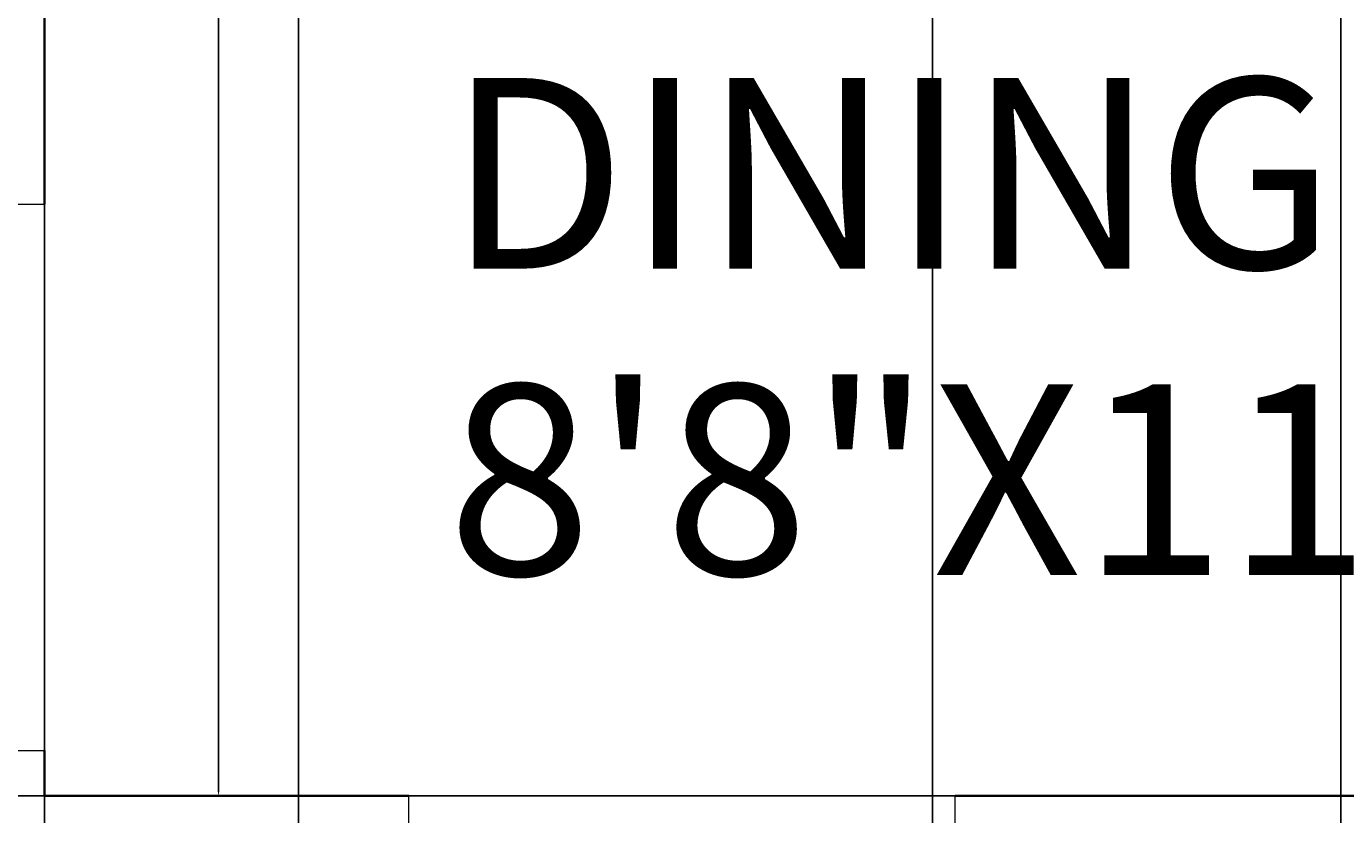
# Model space of a CAD drawing. Units: feet. Extents: x 1654 to 2985, y 1348 to 2230.
# Tile 24 of 53: x 1956 to 2014, y 1750 to 1785. Entities that reach past the tile are written whole.
import ezdxf

# ---------------------------------------------------------------- set-up
doc = ezdxf.new("R2010")
doc.units = ezdxf.units.FT
for name, color, linetype, lineweight in [('A-ANNO-DIMS', 2, 'Continuous', 18), ('A-AREA-IDEN', 7, 'Continuous', 18), ('A-DOOR', 3, 'Continuous', 18), ('A-WALL', 7, 'Continuous', 35)]:
    doc.layers.add(name, color=color, linetype=linetype, lineweight=lineweight)
doc.styles.get("Standard").update_dxf_attribs({"font": 'arial.ttf'})
doc.dimstyles.get("Standard").update_dxf_attribs({"dimtxt": 0.18, "dimasz": 0.18, "dimexe": 0.18, "dimexo": 0.0625, "dimgap": 0.09, "dimtad": 0, "dimtih": 1, "dimtoh": 1, "dimdec": 4, "dimzin": 0, "dimdsep": 46, "dimtxsty": 'Standard', "dimcen": 0.09, "dimadec": 0, "dimazin": 0, "dimtfac": 1, "dimtdec": 4, "dimtofl": 0, "dimtmove": 0, "dimatfit": 3, "dimfxl": 1, "dimtolj": 1, "dimtzin": 0, "dimarcsym": 0})

# ---------------------------------------------------------------- blocks, each defined once
blk = doc.blocks.new('DOOR-INT-SINGLE')
for p, q in [((0, 24), (9, 24)), ((-24, 0), (9, 0))]:
    blk.add_line(p, q)
blk.add_arc((0, 0), 24, 90, 180)
blk = doc.blocks.new('*D74')
at = {"layer": 'A-ANNO-DIMS', "color": 0, "lineweight": -2, "transparency": 16777216}
for p, q in [((1948.155, 1862.255), (1964.922, 1862.255)), ((1964.742, 1862.075), (1964.742, 1806.938)), ((1964.742, 1751.435), (1964.742, 1806.572)), ((1948.155, 1751.255), (1964.922, 1751.255))]:
    blk.add_line(p, q, dxfattribs=at)
at = {"layer": 'A-ANNO-DIMS', "color": 0, "transparency": 16777216}
for points in [[(1964.712, 1862.075), (1964.772, 1862.075), (1964.742, 1862.255)], [(1964.712, 1751.435), (1964.772, 1751.435), (1964.742, 1751.255)]]:
    blk.add_solid(points, dxfattribs=at)
at = {"layer": 'Defpoints', "color": 0, "transparency": 16777216}
for p in [(1948.092, 1862.255), (1964.742, 1862.255), (1948.092, 1751.255)]:
    blk.add_point(p, dxfattribs=at)
at = {"layer": 'A-ANNO-DIMS', "color": 0, "transparency": 16777216, "insert": (1964.742, 1806.755), "char_height": 0.18, "attachment_point": 5}
blk.add_mtext('\\A1;COUNTER 111 TYP.', dxfattribs=at)
blk = doc.blocks.new('*D91')
at = {"layer": 'A-ANNO-DIMS', "color": 0, "lineweight": -2, "transparency": 16777216}
for p, q in [((1852.155, 1801.468), (2242.272, 1801.468)), ((2242.092, 1801.288), (2242.092, 1776.544)), ((2242.092, 1751.435), (2242.092, 1776.18)), ((1852.155, 1751.255), (2242.272, 1751.255))]:
    blk.add_line(p, q, dxfattribs=at)
at = {"layer": 'A-ANNO-DIMS', "color": 0, "transparency": 16777216}
for points in [[(2242.062, 1801.288), (2242.122, 1801.288), (2242.092, 1801.468)], [(2242.062, 1751.435), (2242.122, 1751.435), (2242.092, 1751.255)]]:
    blk.add_solid(points, dxfattribs=at)
at = {"layer": 'Defpoints', "color": 0, "transparency": 16777216}
for p in [(1852.092, 1801.468), (2242.092, 1801.468), (1852.092, 1751.255)]:
    blk.add_point(p, dxfattribs=at)
at = {"layer": 'A-ANNO-DIMS', "color": 0, "transparency": 16777216, "insert": (2242.092, 1776.362), "char_height": 0.18, "attachment_point": 5}
blk.add_mtext('\\A1;50.21', dxfattribs=at)
blk = doc.blocks.new('*D97')
at = {"layer": 'A-ANNO-DIMS', "color": 0, "lineweight": -2, "transparency": 16777216}
for p, q in [((1957.092, 2108.192), (1957.092, 1534.075)), ((1968.254, 2108.192), (1968.254, 1534.075)), ((1957.272, 1534.255), (1962.219, 1534.255)), ((1968.074, 1534.255), (1963.128, 1534.255))]:
    blk.add_line(p, q, dxfattribs=at)
at = {"layer": 'A-ANNO-DIMS', "color": 0, "transparency": 16777216}
for points in [[(1957.272, 1534.285), (1957.272, 1534.225), (1957.092, 1534.255)], [(1968.074, 1534.285), (1968.074, 1534.225), (1968.254, 1534.255)]]:
    blk.add_solid(points, dxfattribs=at)
at = {"layer": 'Defpoints', "color": 0, "transparency": 16777216}
for p in [(1957.092, 2108.255), (1968.254, 2108.255), (1968.254, 1534.255)]:
    blk.add_point(p, dxfattribs=at)
at = {"layer": 'A-ANNO-DIMS', "color": 0, "transparency": 16777216, "insert": (1962.673, 1534.255), "char_height": 0.18, "attachment_point": 5}
blk.add_mtext('\\A1;11.162', dxfattribs=at)
blk = doc.blocks.new('*D98')
at = {"layer": 'A-ANNO-DIMS', "color": 0, "lineweight": -2, "transparency": 16777216}
for p, q in [((2061.03, 1811.081), (1811.912, 1811.081)), ((1812.092, 1810.901), (1812.092, 1781.35)), ((1812.092, 1751.435), (1812.092, 1780.986)), ((2061.03, 1751.255), (1811.912, 1751.255))]:
    blk.add_line(p, q, dxfattribs=at)
at = {"layer": 'A-ANNO-DIMS', "color": 0, "transparency": 16777216}
for points in [[(1812.062, 1810.901), (1812.122, 1810.901), (1812.092, 1811.081)], [(1812.062, 1751.435), (1812.122, 1751.435), (1812.092, 1751.255)]]:
    blk.add_solid(points, dxfattribs=at)
at = {"layer": 'Defpoints', "color": 0, "transparency": 16777216}
for p in [(1812.092, 1811.081), (2061.092, 1811.081), (2061.092, 1751.255)]:
    blk.add_point(p, dxfattribs=at)
at = {"layer": 'A-ANNO-DIMS', "color": 0, "transparency": 16777216, "insert": (1812.092, 1781.168), "char_height": 0.18, "attachment_point": 5}
blk.add_mtext('\\A1;59.83', dxfattribs=at)
blk = doc.blocks.new('*D101')
at = {"layer": 'A-ANNO-DIMS', "color": 0, "lineweight": -2, "transparency": 16777216}
for p, q in [((1996.092, 2039.192), (1996.092, 1534.075)), ((2014.016, 2039.192), (2014.016, 1534.075)), ((1996.272, 1534.255), (2004.599, 1534.255)), ((2013.836, 1534.255), (2005.509, 1534.255))]:
    blk.add_line(p, q, dxfattribs=at)
at = {"layer": 'A-ANNO-DIMS', "color": 0, "transparency": 16777216}
for points in [[(1996.272, 1534.285), (1996.272, 1534.225), (1996.092, 1534.255)], [(2013.836, 1534.285), (2013.836, 1534.225), (2014.016, 1534.255)]]:
    blk.add_solid(points, dxfattribs=at)
at = {"layer": 'Defpoints', "color": 0, "transparency": 16777216}
for p in [(1996.092, 2039.255), (2014.016, 2039.255), (2014.016, 1534.255)]:
    blk.add_point(p, dxfattribs=at)
at = {"layer": 'A-ANNO-DIMS', "color": 0, "transparency": 16777216, "insert": (2005.054, 1534.255), "char_height": 0.18, "attachment_point": 5}
blk.add_mtext('\\A1;17.924', dxfattribs=at)

msp = doc.modelspace()

# ---------------------------------------------------------------- linework, layer by layer
at = {"layer": 'A-WALL'}
for p, q in [((1957.0924, 1777.2549), (1957.0924, 1886.2549)), ((1957.0924, 1751.2549), (1957.0924, 1753.2549)), ((1973.0924, 1751.2549), (1957.0924, 1751.2549)), ((1999.0924, 1751.2549), (1997.0924, 1751.2549)), ((2019.7567, 1751.2549), (1997.0924, 1751.2549))]:
    msp.add_line(p, q, dxfattribs=at)

# ---------------------------------------------------------------- block references
at = {"layer": 'A-DOOR'}
msp.add_blockref('DOOR-INT-SINGLE', (1948.0924, 1753.2549), dxfattribs=at)
at = {"layer": 'A-DOOR', "rotation": 90.00000000000055}
msp.add_blockref('DOOR-INT-SINGLE', (1997.0924, 1742.2549), dxfattribs=at)

# ---------------------------------------------------------------- texts
at = {"layer": 'A-AREA-IDEN'}
for s, p in [('DINING', (1974.793, 1774.4257)), ('8\'8"X11\'3"', (1974.793, 1760.9622))]:
    msp.add_text(s, height=8.38114, dxfattribs=at).set_placement(p)

# ---------------------------------------------------------------- dimensions: what is measured, and where the dimension line sits
at = {"layer": 'A-ANNO-DIMS'}
for base, p1, p2, picture, middle in [((1968.2542, 1534.2549), (1957.0924, 2108.2549), (1968.2542, 2108.2549), '*D97', (1962.6733, 1534.2549)), ((2014.016, 1534.2549), (1996.0924, 2039.2549), (2014.016, 2039.2549), '*D101', (2005.0542, 1534.2549))]:
    dim = msp.add_linear_dim(base=base, p1=p1, p2=p2, dimstyle='Standard', override={"dimdec": 3, "dimlfac": 1, "dimrnd": 0, "dimzin": 0, "dimdsep": 46, "dimlunit": 2}, dxfattribs=at)
    dim.commit()
    dim.dimension.update_dxf_attribs({"geometry": picture, "text_midpoint": middle})
dim = msp.add_linear_dim(base=(1964.7424, 1862.2549), p1=(1948.0924, 1751.2549), p2=(1948.0924, 1862.2549), angle=90, text='COUNTER <> TYP.', dimstyle='Standard', override={"dimdec": 0, "dimlfac": 1, "dimrnd": 0, "dimzin": 0, "dimdsep": 46, "dimlunit": 2}, dxfattribs=at)
dim.commit()
dim.dimension.update_dxf_attribs({"geometry": '*D74', "text_midpoint": (1964.7424, 1806.7549)})
for base, p1, p2, picture, middle in [((1812.0924, 1811.0815), (2061.0924, 1751.2549), (2061.0924, 1811.0815), '*D98', (1812.0924, 1781.1682)), ((2242.0924, 1801.4683), (1852.0924, 1751.2549), (1852.0924, 1801.4683), '*D91', (2242.0924, 1776.3616))]:
    dim = msp.add_linear_dim(base=base, p1=p1, p2=p2, angle=90, dimstyle='Standard', override={"dimdec": 2, "dimlfac": 1, "dimrnd": 0, "dimzin": 0, "dimdsep": 46, "dimlunit": 2}, dxfattribs=at)
    dim.commit()
    dim.dimension.update_dxf_attribs({"geometry": picture, "text_midpoint": middle})

doc.saveas('drawing.dxf')
